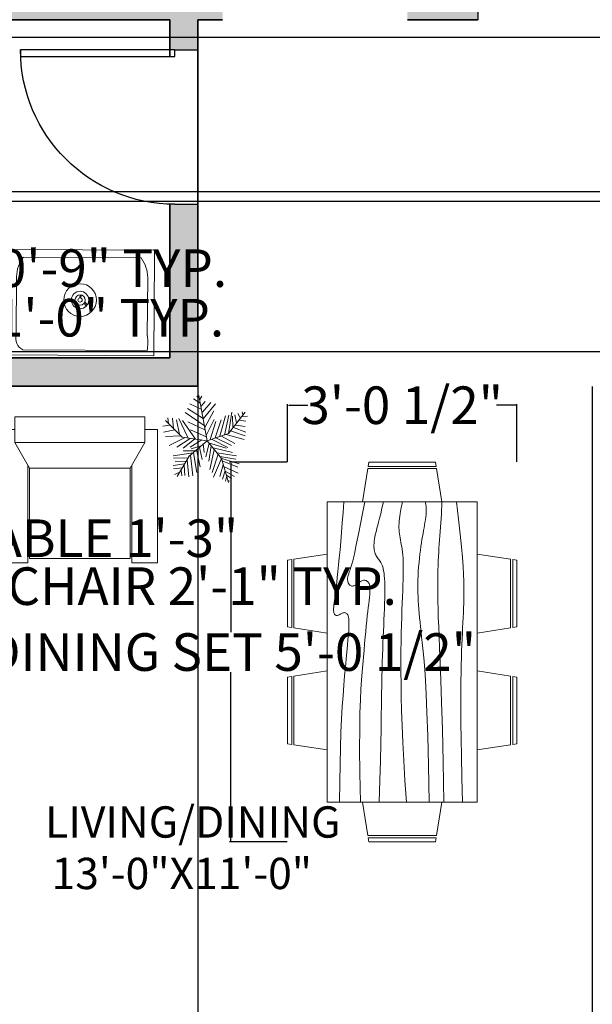
# Model space of a CAD drawing. Units: inches. Extents: x 143233372 to 143233714, y 112671713 to 112672292.
# Tile 3 of 7: x 143233479 to 143233571, y 112671935 to 112672092. Entities that reach past the tile are written whole.
import ezdxf

# ---------------------------------------------------------------- set-up
doc = ezdxf.new("R2010")
doc.units = ezdxf.units.IN
doc.header["$MEASUREMENT"] = 0
doc.layers.get('0').update_dxf_attribs({"color": 104})
for name, color, linetype, lineweight in [('A-ANNO-DIMS', 2, 'Continuous', 18), ('A-AREA-IDEN', 7, 'Continuous', 18), ('doors', 32, 'Continuous', 25), ('furniture', 23, 'Continuous', 18), ('L-PLNT', 92, 'Continuous', 13), ('PLUMBING FIXTURES', 8, 'Continuous', 18), ('walls', 7, 'Continuous', 35)]:
    doc.layers.add(name, color=color, linetype=linetype, lineweight=lineweight)
doc.layers.add('A-WALL-PATT', color=18, linetype='Continuous', lineweight=9, true_color=0x000000)
doc.styles.get("Standard").update_dxf_attribs({"font": 'arial.ttf'})
doc.dimstyles.get("Standard").update_dxf_attribs({"dimtxt": 6, "dimasz": 0.18, "dimexe": 0.18, "dimexo": 0.0625, "dimgap": 0.09, "dimtad": 0, "dimtih": 1, "dimtoh": 1, "dimzin": 0, "dimdsep": 46, "dimlunit": 3, "dimtxsty": 'Standard', "dimcen": 0.09, "dimadec": 0, "dimazin": 0, "dimtfac": 1, "dimtofl": 0, "dimtmove": 0, "dimatfit": 3, "dimfxl": 1, "dimtolj": 1, "dimtzin": 0, "dimarcsym": 0})

# ---------------------------------------------------------------- blocks, each defined once
blk = doc.blocks.new('FABRIC SOFA 1S')
at = {"layer": 'furniture'}
for p, q in [((3, 18.12), (34, 18.12)), ((3, 15.12), (3, 18.12)), ((34, 12.12), (34, 18.12)), ((0, -15.12), (0, 15.12)), ((6, 15.12), (0, 15.12)), ((6, -15.12), (6, 15.12)), ((12, 11.75), (6, 15.12)), ((11.33, 12.12), (34, 12.12)), ((6, -15.12), (12, -11.75)), ((11.33, -12.12), (34, -12.12)), ((34, -12.12), (34, -18.12)), ((6, -15.12), (0, -15.12)), ((3, -18.12), (3, -15.12)), ((3, -18.12), (34, -18.12))]:
    blk.add_line(p, q, dxfattribs=at)
blk.add_lwpolyline([(12, -11.75), (12, 11.75), (33, 11.75), (33, -11.75)], close=True, dxfattribs=at)
blk = doc.blocks.new('Dining Set - 36 x 72 in.')
for p, q in [((-22.2343, 26.00059), (-23.4847, 17.99762)), ((-22.2304, 26), (-5.7608, 26)), ((-22, 27.5), (-22.1562, 26.50042)), ((-5.8416, 26.5), (-22.1534, 26.5)), ((-22, 27.5), (-6, 27.5)), ((-5.8437, 26.49966), (-6, 27.5)), ((-4.5152, 17.99762), (-5.7655, 25.99926)), ((5.7657, 26.00059), (4.5153, 17.99762)), ((5.7696, 26), (22.2392, 26)), ((6, 27.5), (5.8438, 26.50042)), ((22.1584, 26.5), (5.8466, 26.5)), ((6, 27.5), (22, 27.5)), ((22.1563, 26.49966), (22, 27.5)), ((23.4848, 17.99762), (22.2345, 25.99926)), ((36, 18), (-36, 18)), ((-36, 18), (-36, -18)), ((36, -18), (36, 18)), ((-44.0006, 8.23428), (-35.9976, 9.48474)), ((44.0006, 8.23428), (35.9976, 9.48474)), ((-45.5, 8), (-44.5004, 8.15617)), ((-45.5, 8), (-45.5, -8)), ((-44.5, -8.15843), (-44.5, 8.15338)), ((-44, 8.23041), (-44, -8.23915)), ((44, 8.23041), (44, -8.23915)), ((44.5, -8.15843), (44.5, 8.15338)), ((45.5, 8), (44.5005, 8.15617)), ((45.5, 8), (45.5, -8)), ((-44.4997, -8.15631), (-45.5, -8)), ((-35.9976, -9.48476), (-43.9993, -8.2345)), ((35.9976, -9.48476), (43.9993, -8.2345)), ((44.4997, -8.15631), (45.5, -8)), ((-36, -18), (36, -18)), ((-22.2343, -26.0006), (-23.4847, -17.99762)), ((-4.5152, -17.99762), (-5.7655, -25.99928)), ((5.7657, -26.0006), (4.5153, -17.99762)), ((23.4848, -17.99762), (22.2345, -25.99928)), ((-22.2304, -26), (-5.7608, -26)), ((-22, -27.5), (-22.1562, -26.50044)), ((-5.8416, -26.5), (-22.1534, -26.5)), ((-22, -27.5), (-6, -27.5)), ((-5.8437, -26.49967), (-6, -27.5)), ((5.7696, -26), (22.2392, -26)), ((6, -27.5), (5.8438, -26.50044)), ((22.1584, -26.5), (5.8466, -26.5)), ((6, -27.5), (22, -27.5)), ((22.1563, -26.49967), (22, -27.5))]:
    blk.add_line(p, q)
for points in [[(-36, 15), (-31.1772, 14.97754), (-26.8079, 14.91406), (-22.8538, 14.81543), (-19.276, 14.6875), (-16.0362, 14.53613), (-13.0957, 14.36718), (-10.4159, 14.18652), (-7.9583, 14), (-5.6904, 13.81315), (-3.6035, 13.63021), (-1.6954, 13.45508), (0.0365, 13.29166), (1.5945, 13.14388), (2.9811, 13.01562), (4.1988, 12.9108), (5.25, 12.83333), (6.1393, 12.78613), (6.8802, 12.76823), (7.4883, 12.77767), (7.9792, 12.8125), (8.3685, 12.87077), (8.6719, 12.95052), (8.9049, 13.0498), (9.0833, 13.16666), (9.2205, 13.29899), (9.3216, 13.44401), (9.3895, 13.59879), (9.4271, 13.76041), (9.4373, 13.92594), (9.4232, 14.09245), (9.3875, 14.257), (9.3333, 14.41666), (9.2638, 14.56917), (9.1836, 14.71484), (9.0975, 14.85465), (9.0104, 14.98958), (8.9272, 15.1206), (8.8529, 15.2487), (8.7922, 15.37483), (8.75, 15.5), (8.7305, 15.62467), (8.7344, 15.74739), (8.7617, 15.86621), (8.8125, 15.97916), (8.8867, 16.08431), (8.9844, 16.17968), (9.1055, 16.26334), (9.25, 16.33333), (9.4189, 16.38802), (9.6172, 16.42708), (9.8506, 16.45052), (10.125, 16.45833), (10.4463, 16.45052), (10.8203, 16.42708), (11.2529, 16.38802), (11.75, 16.33333), (12.3184, 16.26318), (12.9694, 16.17838), (13.7151, 16.07991), (14.5677, 15.96875), (15.5395, 15.84586), (16.6426, 15.71224), (17.8893, 15.56884), (19.2917, 15.41666), (20.859, 15.25667), (22.5879, 15.08984), (24.4721, 14.91715), (26.5052, 14.73958), (28.6809, 14.5581), (30.9929, 14.3737), (33.4347, 14.18733), (36, 14)], [(-36, 10), (-28.9766, 10.14274), (-23.1725, 10.20442), (-18.4241, 10.19775), (-14.5677, 10.13541), (-11.4399, 10.03011), (-8.877, 9.89453), (-6.7154, 9.74137), (-4.7917, 9.58333), (-2.9698, 9.43082), (-1.2246, 9.28515), (0.4415, 9.14534), (2.026, 9.01041), (3.5266, 8.87939), (4.9408, 8.7513), (6.266, 8.62516), (7.5, 8.5), (8.6411, 8.37549), (9.6914, 8.2539), (10.6538, 8.13818), (11.5312, 8.03125), (12.3267, 7.93603), (13.043, 7.85547), (13.6831, 7.79248), (14.25, 7.75), (14.7471, 7.7303), (15.1797, 7.73307), (15.5537, 7.75732), (15.875, 7.80208), (16.1494, 7.86637), (16.3828, 7.94922), (16.5811, 8.04964), (16.75, 8.16666), (16.8944, 8.29915), (17.0143, 8.44531), (17.1089, 8.60319), (17.1771, 8.77083), (17.218, 8.94629), (17.2305, 9.1276), (17.2137, 9.31282), (17.1667, 9.5), (17.0895, 9.6875), (16.987, 9.875), (16.8649, 10.0625), (16.7292, 10.25), (16.5856, 10.4375), (16.4401, 10.625), (16.2985, 10.8125), (16.1667, 11), (16.05, 11.18733), (15.9518, 11.3737), (15.8752, 11.5581), (15.8229, 11.73958), (15.798, 11.91715), (15.8034, 12.08984), (15.842, 12.25667), (15.9167, 12.41666), (16.0295, 12.56836), (16.1784, 12.70833), (16.3605, 12.83268), (16.5729, 12.9375), (16.8127, 13.01888), (17.0768, 13.07291), (17.3625, 13.0957), (17.6667, 13.08333), (17.9894, 13.03312), (18.3418, 12.94726), (18.7382, 12.82918), (19.1927, 12.68229), (19.7195, 12.51001), (20.3327, 12.31575), (21.0465, 12.10294), (21.875, 11.875), (22.8357, 11.63354), (23.959, 11.37304), (25.2786, 11.08618), (26.8282, 10.76562), (28.6414, 10.40405), (30.752, 9.99414), (33.1936, 9.52856), (36, 9)], [(-36, 5.5), (-30.7157, 5.3348), (-26.069, 5.20963), (-21.9946, 5.11767), (-18.4271, 5.05208), (-15.3009, 5.00602), (-12.5508, 4.97265), (-10.1112, 4.94515), (-7.9167, 4.91666), (-5.909, 4.88167), (-4.0586, 4.83984), (-2.3429, 4.79215), (-0.7396, 4.73958), (0.7739, 4.6831), (2.22, 4.6237), (3.6213, 4.56233), (5, 4.5), (6.373, 4.43782), (7.7344, 4.3776), (9.0723, 4.32129), (10.375, 4.27083), (11.6309, 4.22819), (12.8281, 4.19531), (13.9551, 4.17415), (15, 4.16666), (15.954, 4.17448), (16.819, 4.19791), (17.6001, 4.23698), (18.3021, 4.29166), (18.9299, 4.36198), (19.4883, 4.44791), (19.9823, 4.54948), (20.4167, 4.66666), (20.7969, 4.79899), (21.1302, 4.94401), (21.4245, 5.09879), (21.6875, 5.26041), (21.9271, 5.42594), (22.1511, 5.59245), (22.3672, 5.757), (22.5834, 5.91666), (22.8065, 6.06868), (23.0404, 6.21093), (23.2879, 6.34147), (23.5521, 6.45833), (23.8358, 6.55957), (24.142, 6.64323), (24.4735, 6.70735), (24.8334, 6.75), (25.2235, 6.76969), (25.642, 6.76692), (26.0858, 6.74267), (26.5521, 6.69791), (27.0379, 6.63362), (27.5404, 6.55078), (28.0565, 6.45036), (28.5834, 6.33333), (29.1242, 6.19987), (29.7071, 6.04687), (30.3661, 5.87044), (31.1354, 5.66666), (32.0493, 5.43164), (33.142, 5.16146), (34.4475, 4.85221), (36, 4.5)], [(-36, -1), (-30.7915, -0.6591), (-26.0195, -0.38216), (-21.6519, -0.16284), (-17.6563, 0.00521), (-14.0005, 0.12833), (-10.6523, 0.21289), (-7.5796, 0.26522), (-4.75, 0.29166), (-2.134, 0.29793), (0.2878, 0.28711), (2.5317, 0.26163), (4.6146, 0.22396), (6.5529, 0.17651), (8.3633, 0.12174), (10.0623, 0.06209), (11.6667, 0), (13.1899, -0.06201), (14.6341, -0.1211), (15.9982, -0.17432), (17.2813, -0.21875), (18.4823, -0.25147), (19.6003, -0.26953), (20.6343, -0.27002), (21.5834, -0.25), (22.4481, -0.20768), (23.2357, -0.14584), (23.9549, -0.06836), (24.6146, 0.02083), (25.2235, 0.11784), (25.7904, 0.21875), (26.3241, 0.31966), (26.8334, 0.41666), (27.3265, 0.50618), (27.8099, 0.58593), (28.2894, 0.65397), (28.7709, 0.70833), (29.2601, 0.74707), (29.763, 0.76823), (30.2855, 0.76985), (30.8334, 0.75), (31.4088, 0.70784), (31.9994, 0.64713), (32.589, 0.57275), (33.1615, 0.48958), (33.7008, 0.4025), (34.1908, 0.3164), (34.6153, 0.23616), (34.9584, 0.16666), (35.2099, 0.11165), (35.3848, 0.07031), (35.504, 0.04069), (35.5886, 0.02083), (35.6594, 0.00879), (35.7377, 0.0026), (35.8442, 0.00032), (36, 0)], [(-36, -6.5), (-27.1843, -6.31267), (-20.084, -6.1263), (-14.469, -5.9419), (-10.1094, -5.76042), (-6.7752, -5.58285), (-4.2363, -5.41016), (-2.2629, -5.24333), (-0.625, -5.08334), (0.8708, -4.93099), (2.2715, -4.78646), (3.5872, -4.64974), (4.8281, -4.52084), (6.0046, -4.39974), (7.127, -4.28646), (8.2053, -4.18099), (9.25, -4.08334), (10.2705, -3.99382), (11.2734, -3.91407), (12.2647, -3.84603), (13.25, -3.79167), (14.2354, -3.75293), (15.2266, -3.73177), (16.2295, -3.73015), (17.25, -3.75), (18.2912, -3.79248), (19.3451, -3.85547), (20.4009, -3.93604), (21.4479, -4.03125), (22.4754, -4.13819), (23.4727, -4.25391), (24.4289, -4.37549), (25.3334, -4.5), (26.1785, -4.62492), (26.9694, -4.74935), (27.7145, -4.87281), (28.4219, -4.99479), (29.1, -5.11483), (29.7572, -5.23242), (30.4016, -5.34709), (31.0417, -5.45834), (31.6837, -5.56437), (32.3262, -5.65821), (32.9658, -5.73153), (33.599, -5.77604), (34.2224, -5.78345), (34.8327, -5.74545), (35.4264, -5.65373), (36, -5.5)], [(-36, -10), (-26.4022, -9.81299), (-18.4675, -9.62891), (-11.9839, -9.45069), (-6.7396, -9.28125), (-2.5226, -9.12354), (0.8789, -8.98047), (3.6769, -8.85498), (6.0833, -8.75), (8.2767, -8.66765), (10.3021, -8.60677), (12.1712, -8.56543), (13.8958, -8.54167), (15.4876, -8.53353), (16.9583, -8.53907), (18.3197, -8.55632), (19.5834, -8.58334), (20.7616, -8.61841), (21.8685, -8.66081), (22.9188, -8.71004), (23.9271, -8.76563), (24.9081, -8.82707), (25.8763, -8.89388), (26.8465, -8.96558), (27.8334, -9.04167), (28.8474, -9.12118), (29.8828, -9.20117), (30.93, -9.27824), (31.9792, -9.34896), (33.0205, -9.40991), (34.0443, -9.45768), (35.0407, -9.48885), (36, -9.5)], [(-36, -14.5), (-30.0881, -14.33513), (-25.0332, -14.21224), (-20.7312, -14.12647), (-17.0781, -14.07292), (-13.97, -14.04671), (-11.3027, -14.04297), (-8.9724, -14.05681), (-6.875, -14.08334), (-4.9224, -14.11833), (-3.0905, -14.16016), (-1.3709, -14.20785), (0.2448, -14.26042), (1.7647, -14.3169), (3.1973, -14.3763), (4.5507, -14.43767), (5.8333, -14.5), (7.0554, -14.5621), (8.235, -14.62175), (9.3922, -14.67652), (10.5469, -14.72396), (11.7192, -14.76164), (12.929, -14.78711), (14.1965, -14.79794), (15.5417, -14.79167), (16.9933, -14.76424), (18.6152, -14.70508), (20.4804, -14.60197), (22.6615, -14.44271), (25.2312, -14.21509), (28.2624, -13.9069), (31.8277, -13.50594), (36, -13)]]:
    blk.add_lwpolyline(points)
blk = doc.blocks.new('dining area')
at = {"layer": 'furniture', "xscale": 0.6659924291999282, "yscale": 0.6659924291999282, "zscale": 0.6659924291999282, "rotation": 90}
blk.add_blockref('Dining Set - 36 x 72 in.', (-0.44, 20.51), dxfattribs=at)
blk = doc.blocks.new('*U24')
for p, q in [((0, 0), (0, -6)), ((40, 0), (40, -6))]:
    blk.add_line(p, q)
blk.add_lwpolyline([(0, 0), (0, 40), (1.75, 40), (1.75, 0)], close=True)
blk.add_arc((0, 0), 40, 0, 90)
blk = doc.blocks.new('*U26')
for p, q in [((-8.737, 47.138), (-17.069, 52.711)), ((-10.186, 53.64), (-13.084, 55.962)), ((0, 0), (-10.5, 57)), ((-9.099, 51.782), (-6.563, 55.962)), ((-5.114, 28.097), (-24.676, 40.636)), ((-7.288, 39.707), (-21.778, 46.673)), ((-7.65, 43.423), (-2.578, 49.46)), ((-5.839, 35.992), (4.667, 48.067)), ((-5.114, 27.632), (10.463, 46.673)), ((-2.941, 16.486), (8.652, 37.85)), ((-31.5, 4.5), (-52.5, 25.5)), ((-48.585, 21.131), (-49.309, 29.026)), ((-43.513, 28.561), (-42.427, 15.558)), ((-38.442, 26.239), (-34.819, 7.663)), ((-35.544, 28.097), (-24.314, 3.947)), ((-14.533, 2.09), (-30.834, 25.31)), ((-3.665, 19.273), (-27.574, 35.527)), ((-1.129, 6.734), (9.014, 26.704)), ((10.101, 3.483), (17.708, 26.239)), ((16.259, 5.805), (23.142, 31.348)), ((22.055, 7.198), (27.489, 32.277)), ((27, 9), (48, 36)), ((27.127, 9.056), (31.112, 35.992)), ((31.836, 30.883), (32.561, 16.486)), ((35.096, 32.741), (37.27, 22.524)), ((38.719, 34.134), (41.979, 28.561)), ((40.53, 25.775), (48.862, 24.846)), ((43.791, 29.954), (51.036, 30.883)), ((44.153, 36.456), (45.239, 32.741)), ((-47.498, 19.737), (-55.83, 18.344)), ((-40.615, 13.7), (-55.105, 10.913)), ((-24.314, 23.917), (-2.941, 13.7)), ((-20.691, 13.7), (-1.129, 4.876)), ((3.942, 1.625), (11.187, 24.381)), ((33.285, 16.486), (48.862, 10.913)), ((36.183, 19.737), (48.137, 17.88)), ((-33.37, 6.269), (-52.207, 5.34)), ((-28.299, 3.483), (-47.86, -5.805)), ((-21.416, 3.018), (-38.079, -8.128)), ((0, 0), (-31.5, 4.5)), ((-15.982, 2.09), (-30.11, -9.521)), ((0, 0), (-22.5, -19.5)), ((-6.563, 1.161), (-21.416, -8.128)), ((0, 0), (27, 9)), ((0, 0), (18, -22.5)), ((6.478, 1.625), (26.04, -8.592)), ((11.187, 3.483), (30.749, -5.805)), ((18.07, 5.805), (35.096, -3.483)), ((24.229, 7.663), (46.688, 1.625)), ((29.662, 12.307), (48.137, 6.269)), ((-6.563, -5.805), (-19.967, -9.985)), ((-13.446, -11.378), (-8.737, -32.741)), ((-9.461, -8.592), (-6.201, -23.453)), ((-4.752, -3.483), (-3.665, -14.629)), ((2.493, -3.019), (-1.491, -20.202)), ((1.769, -2.555), (24.229, -9.521)), ((5.029, -6.27), (2.131, -25.775)), ((9.014, -11.378), (3.58, -35.992)), ((7.565, -9.056), (32.198, -14.629)), ((-17.431, -15.094), (-42.789, -18.809)), ((-24.314, -21.596), (-42.427, -22.06)), ((-22.5, -19.5), (-37.5, -45)), ((-15.257, -12.772), (-30.11, -12.772)), ((-25.038, -23.918), (-22.865, -45.281)), ((-20.691, -18.345), (-17.793, -44.352)), ((-17.069, -15.094), (-12.721, -40.172)), ((14.085, -16.951), (6.478, -40.172)), ((18.07, -22.524), (8.289, -45.745)), ((12.274, -15.094), (36.907, -18.809)), ((16.259, -19.738), (36.183, -22.989)), ((18, -22.5), (27, -52.5)), ((18.433, -22.524), (40.53, -29.026)), ((-28.299, -29.026), (-42.789, -31.348)), ((-30.834, -34.135), (-42.427, -35.528)), ((-26.849, -26.24), (-40.253, -25.775)), ((-32.646, -36.921), (-31.921, -44.352)), ((-29.023, -30.884), (-27.936, -43.887)), ((20.244, -30.419), (15.897, -44.816)), ((19.157, -25.311), (38.719, -33.206)), ((21.331, -32.741), (39.081, -40.636)), ((-34.457, -39.708), (-40.978, -42.494)), ((22.78, -37.85), (19.519, -48.532)), ((22.78, -38.314), (34.372, -44.816)), ((24.591, -45.745), (23.142, -50.854)), ((24.591, -43.423), (30.749, -47.603)), ((26.764, -49.925), (28.213, -50.854))]:
    blk.add_line(p, q)
blk = doc.blocks.new('LAVATORY-RECT')
for p, q in [((0, 0.15), (0.11, 17)), ((0.11, 17), (23.11, 16.85)), ((20.97, 15.65), (2.15, 15.77)), ((23.11, 16.85), (23.1, 15.71)), ((23.1, 15.71), (23, 0)), ((0.99, 3.35), (1.05, 12.64)), ((21.96, 3.21), (22.03, 12.5)), ((11.22, 9.73), (11.16, 9.24)), ((11.36, 9.22), (11.4, 9.7)), ((10.4, 8.91), (9.84, 8.81)), ((10.52, 8.7), (9.87, 8.58)), ((11.84, 8.39), (12.22, 7.95)), ((11.97, 8.6), (12.36, 8.13)), ((23, 0), (0, 0.15)), ((21.95, 0.84), (2.06, 0.97))]:
    blk.add_line(p, q)
for radius in [2.61, 1.39, 0.816, 0.338]:
    blk.add_circle((11.22, 8.91), radius)
for centre, radius, start, end in [((6.46, 12.5), 5.4, 142.7525, 178.5493), ((16.62, 12.43), 5.4, 0.6949, 36.4918), ((3, 2.82), 2.08, 165.2338, 242.9258), ((12.7, 2.09), 9.33, 352.3124, 6.9318)]:
    blk.add_arc(centre, radius, start, end)
blk = doc.blocks.new('*D35')
at = {"layer": 'A-ANNO-DIMS', "color": 0, "lineweight": -2, "transparency": 16777216}
for p, q in [((143233450.89, 112672004.93), (143233450.89, 112672001.08)), ((143233475.74, 112672004.93), (143233475.74, 112672001.08)), ((143233451.07, 112672001.26), (143233475.56, 112672001.26)), ((143233475.74, 112672001.26), (143233475.92, 112672001.26))]:
    blk.add_line(p, q, dxfattribs=at)
at = {"layer": 'A-ANNO-DIMS', "color": 0, "transparency": 16777216}
for points in [[(143233451.07, 112672001.29), (143233451.07, 112672001.23), (143233450.89, 112672001.26)], [(143233475.56, 112672001.29), (143233475.56, 112672001.23), (143233475.74, 112672001.26)]]:
    blk.add_solid(points, dxfattribs=at)
at = {"layer": 'Defpoints', "color": 0, "transparency": 16777216}
for p in [(143233450.89, 112672004.99), (143233475.74, 112672004.99), (143233475.74, 112672001.26)]:
    blk.add_point(p, dxfattribs=at)
at = {"layer": 'A-ANNO-DIMS', "color": 0, "transparency": 16777216, "insert": (143233508.46, 112672001.26), "char_height": 6, "attachment_point": 5}
blk.add_mtext('\\A1;CHAIR 2\'-1" TYP.', dxfattribs=at)
blk = doc.blocks.new('*D49')
at = {"layer": 'A-ANNO-DIMS', "color": 0, "lineweight": -2, "transparency": 16777216}
for p, q in [((143233475.63, 112672050.2), (143233477.58, 112672050.2)), ((143233477.4, 112672050.02), (143233477.4, 112672047.31)), ((143233477.4, 112672038.21), (143233477.4, 112672040.92)), ((143233475.63, 112672038.03), (143233477.58, 112672038.03))]:
    blk.add_line(p, q, dxfattribs=at)
at = {"layer": 'A-ANNO-DIMS', "color": 0, "transparency": 16777216}
for points in [[(143233477.37, 112672050.02), (143233477.43, 112672050.02), (143233477.4, 112672050.2)], [(143233477.37, 112672038.21), (143233477.43, 112672038.21), (143233477.4, 112672038.03)]]:
    blk.add_solid(points, dxfattribs=at)
at = {"layer": 'Defpoints', "color": 0, "transparency": 16777216}
for p in [(143233475.57, 112672050.2), (143233475.57, 112672038.03), (143233477.4, 112672038.03)]:
    blk.add_point(p, dxfattribs=at)
at = {"layer": 'A-ANNO-DIMS', "color": 0, "transparency": 16777216, "insert": (143233477.4, 112672044.11), "char_height": 6, "attachment_point": 5}
blk.add_mtext('\\A1;FITTING 1\'-0" TYP.', dxfattribs=at)
blk = doc.blocks.new('*D50')
at = {"layer": 'A-ANNO-DIMS', "color": 0, "lineweight": -2, "transparency": 16777216}
for p, q in [((143233466.57, 112672050.26), (143233466.57, 112672052.2)), ((143233466.75, 112672052.02), (143233475.39, 112672052.02)), ((143233475.57, 112672050.26), (143233475.57, 112672052.2)), ((143233475.57, 112672052.02), (143233475.75, 112672052.02))]:
    blk.add_line(p, q, dxfattribs=at)
at = {"layer": 'A-ANNO-DIMS', "color": 0, "transparency": 16777216}
for points in [[(143233466.75, 112672052.05), (143233466.75, 112672051.99), (143233466.57, 112672052.02)], [(143233475.39, 112672052.05), (143233475.39, 112672051.99), (143233475.57, 112672052.02)]]:
    blk.add_solid(points, dxfattribs=at)
at = {"layer": 'Defpoints', "color": 0, "transparency": 16777216}
for p in [(143233475.57, 112672052.02), (143233466.57, 112672050.2), (143233475.57, 112672050.2)]:
    blk.add_point(p, dxfattribs=at)
at = {"layer": 'A-ANNO-DIMS', "color": 0, "transparency": 16777216, "insert": (143233494.13, 112672052.02), "char_height": 6, "attachment_point": 5}
blk.add_mtext('\\A1;0\'-9" TYP.', dxfattribs=at)
blk = doc.blocks.new('*D55')
at = {"layer": 'A-ANNO-DIMS', "color": 0, "lineweight": -2, "transparency": 16777216}
for p, q in [((143233433.65, 112672011.09), (143233433.65, 112672008.73)), ((143233448.6, 112672011.09), (143233448.6, 112672008.73)), ((143233433.83, 112672008.91), (143233448.42, 112672008.91)), ((143233448.6, 112672008.91), (143233448.78, 112672008.91))]:
    blk.add_line(p, q, dxfattribs=at)
at = {"layer": 'A-ANNO-DIMS', "color": 0, "transparency": 16777216}
for points in [[(143233433.83, 112672008.94), (143233433.83, 112672008.88), (143233433.65, 112672008.91)], [(143233448.42, 112672008.94), (143233448.42, 112672008.88), (143233448.6, 112672008.91)]]:
    blk.add_solid(points, dxfattribs=at)
at = {"layer": 'Defpoints', "color": 0, "transparency": 16777216}
for p in [(143233433.65, 112672011.15), (143233448.6, 112672011.15), (143233448.6, 112672008.91)]:
    blk.add_point(p, dxfattribs=at)
at = {"layer": 'A-ANNO-DIMS', "color": 0, "transparency": 16777216, "insert": (143233482.22, 112672008.91), "char_height": 6, "attachment_point": 5}
blk.add_mtext('\\A1;SIDE TABLE 1\'-3"', dxfattribs=at)
blk = doc.blocks.new('*D61')
at = {"layer": 'A-ANNO-DIMS', "color": 0, "lineweight": -2, "transparency": 16777216}
for p, q in [((143233522.04, 112672021.05), (143233512.83, 112672021.05)), ((143233513.01, 112672020.87), (143233513.01, 112671993.94)), ((143233513.01, 112671960.62), (143233513.01, 112671987.55)), ((143233522.04, 112671960.44), (143233512.83, 112671960.44))]:
    blk.add_line(p, q, dxfattribs=at)
at = {"layer": 'A-ANNO-DIMS', "color": 0, "transparency": 16777216}
for points in [[(143233512.98, 112672020.87), (143233513.04, 112672020.87), (143233513.01, 112672021.05)], [(143233512.98, 112671960.62), (143233513.04, 112671960.62), (143233513.01, 112671960.44)]]:
    blk.add_solid(points, dxfattribs=at)
at = {"layer": 'Defpoints', "color": 0, "transparency": 16777216}
for p in [(143233513.01, 112672021.05), (143233522.1, 112672021.05), (143233522.1, 112671960.44)]:
    blk.add_point(p, dxfattribs=at)
at = {"layer": 'A-ANNO-DIMS', "color": 0, "transparency": 16777216, "insert": (143233513.01, 112671990.74), "char_height": 6, "attachment_point": 5}
blk.add_mtext('\\A1;DINING SET 5\'-0 1/2"', dxfattribs=at)
blk = doc.blocks.new('*D62')
at = {"layer": 'A-ANNO-DIMS', "color": 0, "lineweight": -2, "transparency": 16777216}
for p, q in [((143233522.1, 112672021.11), (143233522.1, 112672030.32)), ((143233522.28, 112672030.14), (143233525.36, 112672030.14)), ((143233558.55, 112672030.14), (143233555.47, 112672030.14)), ((143233558.73, 112672021.11), (143233558.73, 112672030.32))]:
    blk.add_line(p, q, dxfattribs=at)
at = {"layer": 'A-ANNO-DIMS', "color": 0, "transparency": 16777216}
for points in [[(143233522.28, 112672030.17), (143233522.28, 112672030.11), (143233522.1, 112672030.14)], [(143233558.55, 112672030.17), (143233558.55, 112672030.11), (143233558.73, 112672030.14)]]:
    blk.add_solid(points, dxfattribs=at)
at = {"layer": 'Defpoints', "color": 0, "transparency": 16777216}
for p in [(143233558.73, 112672030.14), (143233522.1, 112672021.05), (143233558.73, 112672021.05)]:
    blk.add_point(p, dxfattribs=at)
at = {"layer": 'A-ANNO-DIMS', "color": 0, "transparency": 16777216, "insert": (143233540.41, 112672030.14), "char_height": 6, "attachment_point": 5}
blk.add_mtext('\\A1;3\'-0 1/2"', dxfattribs=at)
blk = doc.blocks.new('*D69')
at = {"layer": 'A-ANNO-DIMS', "color": 0, "lineweight": -2, "transparency": 16777216}
for p, q in [((143233507.78, 112672033.12), (143233507.78, 112671717.12)), ((143233570.78, 112672033.12), (143233570.78, 112671717.12)), ((143233507.96, 112671717.3), (143233531.22, 112671717.3)), ((143233570.6, 112671717.3), (143233547.35, 112671717.3))]:
    blk.add_line(p, q, dxfattribs=at)
at = {"layer": 'A-ANNO-DIMS', "color": 0, "transparency": 16777216}
for points in [[(143233507.96, 112671717.33), (143233507.96, 112671717.27), (143233507.78, 112671717.3)], [(143233570.6, 112671717.33), (143233570.6, 112671717.27), (143233570.78, 112671717.3)]]:
    blk.add_solid(points, dxfattribs=at)
at = {"layer": 'Defpoints', "color": 0, "transparency": 16777216}
for p in [(143233507.78, 112672033.18), (143233570.78, 112672033.18), (143233570.78, 112671717.3)]:
    blk.add_point(p, dxfattribs=at)
at = {"layer": 'A-ANNO-DIMS', "color": 0, "transparency": 16777216, "insert": (143233539.28, 112671717.3), "char_height": 6, "attachment_point": 5}
blk.add_mtext('\\A1;5\'-3"', dxfattribs=at)
blk = doc.blocks.new('*D70')
at = {"layer": 'A-ANNO-DIMS', "color": 0, "lineweight": -2, "transparency": 16777216}
for p, q in [((143233574.42, 112672088.85), (143233389.09, 112672088.85)), ((143233389.27, 112672088.67), (143233389.27, 112672079.72)), ((143233389.27, 112672064.38), (143233389.27, 112672073.33)), ((143233575.22, 112672064.2), (143233389.09, 112672064.2))]:
    blk.add_line(p, q, dxfattribs=at)
at = {"layer": 'A-ANNO-DIMS', "color": 0, "transparency": 16777216}
for points in [[(143233389.24, 112672088.67), (143233389.3, 112672088.67), (143233389.27, 112672088.85)], [(143233389.24, 112672064.38), (143233389.3, 112672064.38), (143233389.27, 112672064.2)]]:
    blk.add_solid(points, dxfattribs=at)
at = {"layer": 'Defpoints', "color": 0, "transparency": 16777216}
for p in [(143233574.48, 112672088.85), (143233389.27, 112672064.2), (143233575.28, 112672064.2)]:
    blk.add_point(p, dxfattribs=at)
at = {"layer": 'A-ANNO-DIMS', "color": 0, "transparency": 16777216, "insert": (143233389.27, 112672076.53), "char_height": 6, "attachment_point": 5}
blk.add_mtext('\\A1;2\'-0 1/2"', dxfattribs=at)
blk = doc.blocks.new('*D72')
at = {"layer": 'A-ANNO-DIMS', "color": 0, "lineweight": -2, "transparency": 16777216}
for p, q in [((143233576.46, 112672062.68), (143233389.09, 112672062.68)), ((143233389.27, 112672062.5), (143233389.27, 112672053.84)), ((143233389.27, 112672038.86), (143233389.27, 112672047.53)), ((143233586.96, 112672038.68), (143233389.09, 112672038.68))]:
    blk.add_line(p, q, dxfattribs=at)
at = {"layer": 'A-ANNO-DIMS', "color": 0, "transparency": 16777216}
for points in [[(143233389.24, 112672062.5), (143233389.3, 112672062.5), (143233389.27, 112672062.68)], [(143233389.24, 112672038.86), (143233389.3, 112672038.86), (143233389.27, 112672038.68)]]:
    blk.add_solid(points, dxfattribs=at)
at = {"layer": 'Defpoints', "color": 0, "transparency": 16777216}
for p in [(143233576.53, 112672062.68), (143233389.27, 112672038.68), (143233587.03, 112672038.68)]:
    blk.add_point(p, dxfattribs=at)
at = {"layer": 'A-ANNO-DIMS', "color": 0, "transparency": 16777216, "insert": (143233389.27, 112672050.68), "char_height": 6, "attachment_point": 5}
blk.add_mtext('\\A1;2\'-0"', dxfattribs=at)

msp = doc.modelspace()

# ---------------------------------------------------------------- hatches: boundary and pattern name
at = {"layer": 'A-WALL-PATT'}
h = msp.add_hatch(color=256, dxfattribs=at)
h.dxf.hatch_style = 1
h.paths.add_polyline_path([(143233549.785, 112672240.182), (143233545.285, 112672240.182), (143233545.285, 112672096.182), (143233541.241, 112672096.182), (143233541.241, 112672091.682), (143233552.476, 112672091.682), (143233552.476, 112672096.182), (143233549.785, 112672096.182)])
h = msp.add_hatch(color=256, dxfattribs=at)
h.dxf.hatch_style = 1
h.paths.add_polyline_path([(143233507.785, 112672062.229), (143233504.087, 112672062.229, -0.0081431), (143233503.285, 112672062.242), (143233503.285, 112672037.682), (143233425.285, 112672037.682), (143233425.285, 112672033.182), (143233507.785, 112672033.182)])
h.paths.add_polyline_path([(143233511.719, 112672096.182), (143233425.285, 112672096.182), (143233425.285, 112672091.682), (143233503.285, 112672091.682), (143233503.285, 112672086.878), (143233504.087, 112672086.878), (143233507.785, 112672086.878), (143233507.785, 112672091.682), (143233511.719, 112672091.682)])

# ---------------------------------------------------------------- linework, layer by layer
at = {"layer": 'walls'}
for p, q in [((143233425.285, 112672091.682), (143233503.285, 112672091.682)), ((143233503.285, 112672085.8), (143233503.285, 112672091.682)), ((143233507.785, 112672033.182), (143233507.785, 112672091.682)), ((143233507.785, 112672091.682), (143233511.719, 112672091.682)), ((143233541.241, 112672091.682), (143233552.476, 112672091.682)), ((143233503.285, 112672037.682), (143233503.285, 112672062.242)), ((143233425.285, 112672037.682), (143233503.285, 112672037.682)), ((143233425.285, 112672033.182), (143233507.785, 112672033.182))]:
    msp.add_line(p, q, dxfattribs=at)

# ---------------------------------------------------------------- block references
at = {"layer": 'doors', "xscale": 0.7380496403518878, "yscale": 0.7380496403518878, "zscale": 0.7380496403518878}
msp.add_blockref('*U24', (143233552.476, 112672096.111), dxfattribs=at)
at = {"layer": 'doors', "xscale": -0.6162162669326948, "yscale": 0.6162162669326948, "zscale": 0.6162162669326948, "rotation": 90}
msp.add_blockref('*U24', (143233504.087, 112672086.878), dxfattribs=at)
at = {"layer": 'furniture', "xscale": 0.685544738852578, "yscale": 0.685544738852578, "zscale": 0.685544738852578, "rotation": 270}
msp.add_blockref('FABRIC SOFA 1S', (143233488.92, 112672028.298), dxfattribs=at)
at = {"layer": 'furniture'}
msp.add_blockref('dining area', (143233540.851, 112671970.238), dxfattribs=at)
at = {"layer": 'L-PLNT', "xscale": 0.1267628913715484, "yscale": 0.1267628913715484, "zscale": 0.1267628913715484}
msp.add_blockref('*U26', (143233509.24, 112672024.47), dxfattribs=at)
at = {"layer": 'PLUMBING FIXTURES'}
msp.add_blockref('LAVATORY-RECT', (143233477.735, 112672038.024), dxfattribs=at)

# ---------------------------------------------------------------- texts
at = {"layer": 'A-AREA-IDEN'}
for s, p in [('LIVING/DINING', (143233483.373, 112671961.114)), ('13\'-0"X11\'-0"', (143233484.39, 112671952.9))]:
    msp.add_text(s, height=5, dxfattribs=at).set_placement(p)

# ---------------------------------------------------------------- dimensions: what is measured, and where the dimension line sits
at = {"layer": 'A-ANNO-DIMS'}
for base, p1, p2, picture, middle in [((143233389.272, 112672064.202), (143233574.482, 112672088.851), (143233575.285, 112672064.202), '*D70', (143233389.272, 112672076.526)), ((143233389.272, 112672038.682), (143233576.526, 112672062.682), (143233587.026, 112672038.682), '*D72', (143233389.272, 112672050.682))]:
    dim = msp.add_linear_dim(base=base, p1=p1, p2=p2, angle=90, dimstyle='Standard', override={"dimdec": 1, "dimlfac": 1, "dimrnd": 0, "dimzin": 1, "dimdsep": 46, "dimlunit": 4, "dimfrac": 2}, dxfattribs=at)
    dim.commit()
    dim.dimension.update_dxf_attribs({"geometry": picture, "text_midpoint": middle})
for base, p1, p2, text, picture, middle in [((143233475.571, 112672052.023), (143233466.571, 112672050.197), (143233475.571, 112672050.197), '<> TYP.', '*D50', (143233494.128, 112672052.023)), ((143233448.599, 112672008.907), (143233433.654, 112672011.149), (143233448.599, 112672011.149), 'SIDE TABLE <>', '*D55', (143233482.217, 112672008.907)), ((143233475.738, 112672001.261), (143233450.887, 112672004.989), (143233475.738, 112672004.989), 'CHAIR <> TYP.', '*D35', (143233508.463, 112672001.261))]:
    dim = msp.add_linear_dim(base=base, p1=p1, p2=p2, text=text, dimstyle='Standard', override={"dimdec": 1, "dimlfac": 1, "dimrnd": 0, "dimzin": 1, "dimdsep": 46, "dimlunit": 4, "dimfrac": 2}, dxfattribs=at)
    dim.commit()
    dim.dimension.update_dxf_attribs({"geometry": picture, "text_midpoint": middle})
for base, p1, p2, angle, text, picture, middle in [((143233477.396, 112672038.029), (143233475.571, 112672050.197), (143233475.571, 112672038.029), 270, 'FITTING <> TYP.', '*D49', (143233477.396, 112672044.113)), ((143233513.007, 112672021.047), (143233522.098, 112671960.442), (143233522.098, 112672021.047), 90, 'DINING SET <>', '*D61', (143233513.007, 112671990.745))]:
    dim = msp.add_linear_dim(base=base, p1=p1, p2=p2, angle=angle, text=text, dimstyle='Standard', override={"dimdec": 1, "dimlfac": 1, "dimrnd": 0, "dimzin": 1, "dimdsep": 46, "dimlunit": 4, "dimfrac": 2}, dxfattribs=at)
    dim.commit()
    dim.dimension.update_dxf_attribs({"geometry": picture, "text_midpoint": middle})
for base, p1, p2, picture, middle in [((143233558.727, 112672030.138), (143233522.098, 112672021.047), (143233558.727, 112672021.047), '*D62', (143233540.413, 112672030.138)), ((143233570.785, 112671717.299), (143233507.785, 112672033.182), (143233570.785, 112672033.182), '*D69', (143233539.285, 112671717.299))]:
    dim = msp.add_linear_dim(base=base, p1=p1, p2=p2, dimstyle='Standard', override={"dimdec": 1, "dimlfac": 1, "dimrnd": 0, "dimzin": 1, "dimdsep": 46, "dimlunit": 4, "dimfrac": 2}, dxfattribs=at)
    dim.commit()
    dim.dimension.update_dxf_attribs({"geometry": picture, "text_midpoint": middle})

doc.saveas('drawing.dxf')
